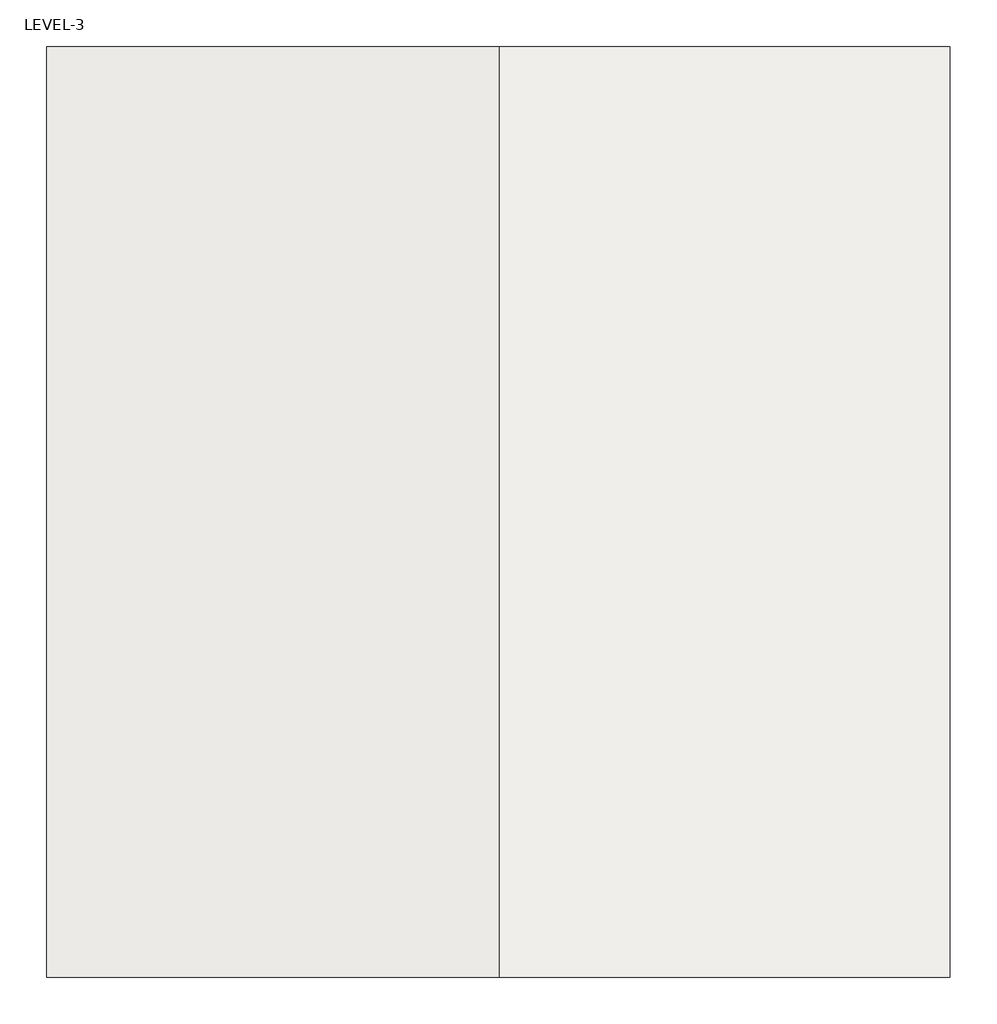
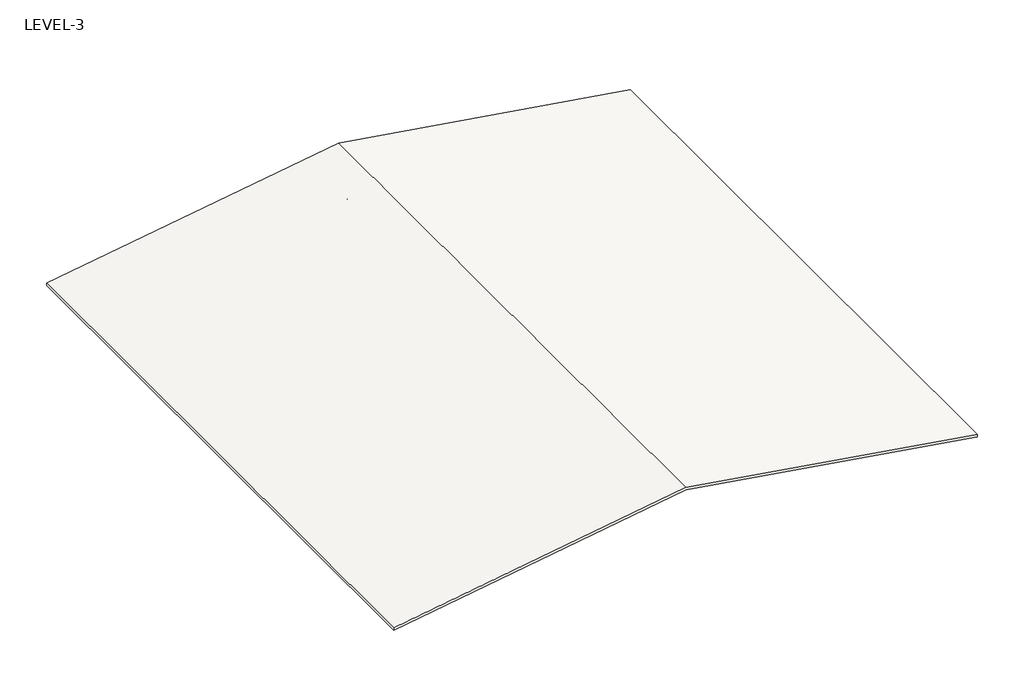
# One storey: 24 beams, 1 roof.
"""IFC4 building model written with IfcOpenShell, lengths in millimetres."""

from ifc_helpers import new_model, si_unit, frame, origin, place, context, project, spatial, polyline, outline, extrude, transform, mapped, element, save
from components import ub_universal_beams_ub305x165x40_7500c72c, ub_universal_beams_ub305x165x40_0b90c1cb, ub_universal_beams_ub305x165x40_52a2f76b, ub_universal_beams_ub305x165x40_7a055ae5

model = new_model("IFC4")

# Units and contexts
model_context = context("Model", 3, world=origin())
ifc_project = project(units=[si_unit("LENGTHUNIT", "METRE", prefix="MILLI")], contexts=[model_context])

# Site, building, storey
site = spatial("IfcSite", under=ifc_project)
building = spatial("IfcBuilding", under=site)
storey = spatial("IfcBuildingStorey", under=building, Name="LEVEL-3", Elevation=6706.0)

# Beams
placement = place(None, origin())
ub_universal_beams_ub305x165x40_shape = ub_universal_beams_ub305x165x40_7500c72c(model_context)
element("IfcBeam", 1, ObjectType="UB-Universal Beams : UB305x165x40", at=placement, inside=storey, context=model_context, shape_type="MappedRepresentation", body=[
    mapped(ub_universal_beams_ub305x165x40_shape, transform((-6850.9138812, -14328.4765895, 5828.2801742), x_axis=(1.0, 0.0, 0.0), y_axis=(0.0, -1.0, 0.0), z_axis=(0.0, 0.0, -1.0))),
])
element("IfcBeam", 2, ObjectType="UB-Universal Beams : UB305x165x40", at=placement, inside=storey, context=model_context, shape_type="MappedRepresentation", body=[
    mapped(ub_universal_beams_ub305x165x40_shape, transform((-6850.9138812, -8232.4765895, 5828.2801742), x_axis=(1.0, 0.0, 0.0), y_axis=(0.0, -1.0, 0.0), z_axis=(0.0, 0.0, -1.0))),
])
element("IfcBeam", 3, ObjectType="UB-Universal Beams : UB305x165x40", at=placement, inside=storey, context=model_context, shape_type="MappedRepresentation", body=[
    mapped(ub_universal_beams_ub305x165x40_shape, transform((-6850.9138812, -2136.4765895, 5828.2801742), x_axis=(1.0, 0.0, 0.0), y_axis=(0.0, -1.0, 0.0), z_axis=(0.0, 0.0, -1.0))),
])
element("IfcBeam", 4, ObjectType="UB-Universal Beams : UB305x165x40", at=placement, inside=storey, context=model_context, shape_type="MappedRepresentation", body=[
    mapped(ub_universal_beams_ub305x165x40_shape, transform((-6850.9138812, 3959.5234105, 5828.2801742), x_axis=(1.0, 0.0, 0.0), y_axis=(0.0, -1.0, 0.0), z_axis=(0.0, 0.0, -1.0))),
])
element("IfcBeam", 5, ObjectType="UB-Universal Beams : UB305x165x40", at=placement, inside=storey, context=model_context, shape_type="MappedRepresentation", body=[
    mapped(ub_universal_beams_ub305x165x40_shape, transform((-6850.9138812, 10055.5234105, 5828.2801742), x_axis=(1.0, 0.0, 0.0), y_axis=(0.0, -1.0, 0.0), z_axis=(0.0, 0.0, -1.0))),
])
element("IfcBeam", 6, ObjectType="UB-Universal Beams : UB305x165x40", at=placement, inside=storey, context=model_context, shape_type="MappedRepresentation", body=[
    mapped(ub_universal_beams_ub305x165x40_shape, transform((-6850.9138812, 16151.5234105, 5828.2801742), x_axis=(1.0, 0.0, 0.0), y_axis=(0.0, -1.0, 0.0), z_axis=(0.0, 0.0, -1.0))),
])
ub_universal_beams_ub305x165x40_2_shape = ub_universal_beams_ub305x165x40_0b90c1cb(model_context)
element("IfcBeam", 7, ObjectType="UB-Universal Beams : UB305x165x40", at=placement, inside=storey, context=model_context, shape_type="MappedRepresentation", body=[
    mapped(ub_universal_beams_ub305x165x40_2_shape, transform((250.2473103, -14328.4765895, 5828.2801742), x_axis=(1.0, 0.0, 0.0), y_axis=(0.0, -1.0, 0.0), z_axis=(0.0, 0.0, -1.0))),
])
element("IfcBeam", 8, ObjectType="UB-Universal Beams : UB305x165x40", at=placement, inside=storey, context=model_context, shape_type="MappedRepresentation", body=[
    mapped(ub_universal_beams_ub305x165x40_2_shape, transform((250.2473103, -8232.4765895, 5828.2801742), x_axis=(1.0, 0.0, 0.0), y_axis=(0.0, -1.0, 0.0), z_axis=(0.0, 0.0, -1.0))),
])
element("IfcBeam", 9, ObjectType="UB-Universal Beams : UB305x165x40", at=placement, inside=storey, context=model_context, shape_type="MappedRepresentation", body=[
    mapped(ub_universal_beams_ub305x165x40_2_shape, transform((250.2473103, -2136.4765895, 5828.2801742), x_axis=(1.0, 0.0, 0.0), y_axis=(0.0, -1.0, 0.0), z_axis=(0.0, 0.0, -1.0))),
])
element("IfcBeam", 10, ObjectType="UB-Universal Beams : UB305x165x40", at=placement, inside=storey, context=model_context, shape_type="MappedRepresentation", body=[
    mapped(ub_universal_beams_ub305x165x40_2_shape, transform((250.2473103, 3959.5234105, 5828.2801742), x_axis=(1.0, 0.0, 0.0), y_axis=(0.0, -1.0, 0.0), z_axis=(0.0, 0.0, -1.0))),
])
element("IfcBeam", 11, ObjectType="UB-Universal Beams : UB305x165x40", at=placement, inside=storey, context=model_context, shape_type="MappedRepresentation", body=[
    mapped(ub_universal_beams_ub305x165x40_2_shape, transform((250.2473103, 10055.5234105, 5828.2801742), x_axis=(1.0, 0.0, 0.0), y_axis=(0.0, -1.0, 0.0), z_axis=(0.0, 0.0, -1.0))),
])
element("IfcBeam", 12, ObjectType="UB-Universal Beams : UB305x165x40", at=placement, inside=storey, context=model_context, shape_type="MappedRepresentation", body=[
    mapped(ub_universal_beams_ub305x165x40_2_shape, transform((250.2473103, 16151.5234105, 5828.2801742), x_axis=(1.0, 0.0, 0.0), y_axis=(0.0, -1.0, 0.0), z_axis=(0.0, 0.0, -1.0))),
])
ub_universal_beams_ub305x165x40_3_shape = ub_universal_beams_ub305x165x40_52a2f76b(model_context)
element("IfcBeam", 13, ObjectType="UB-Universal Beams : UB305x165x40", at=placement, inside=storey, context=model_context, shape_type="MappedRepresentation", body=[
    mapped(ub_universal_beams_ub305x165x40_3_shape, transform((-5118.5854152, -14328.4765895, 6101.0878067), x_axis=(0.15556314184436565, 0.0, -0.9878259507117181), y_axis=(0.0, -1.0, 0.0), z_axis=(-0.9878259507117181, 0.0, -0.15556314184436565))),
])
element("IfcBeam", 14, ObjectType="UB-Universal Beams : UB305x165x40", at=placement, inside=storey, context=model_context, shape_type="MappedRepresentation", body=[
    mapped(ub_universal_beams_ub305x165x40_3_shape, transform((-5118.5854152, -8232.4765895, 6101.0878067), x_axis=(0.15556314184436565, 0.0, -0.9878259507117181), y_axis=(0.0, -1.0, 0.0), z_axis=(-0.9878259507117181, 0.0, -0.15556314184436565))),
])
element("IfcBeam", 15, ObjectType="UB-Universal Beams : UB305x165x40", at=placement, inside=storey, context=model_context, shape_type="MappedRepresentation", body=[
    mapped(ub_universal_beams_ub305x165x40_3_shape, transform((-5118.5854152, -2136.4765895, 6101.0878067), x_axis=(0.15556314184436565, 0.0, -0.9878259507117181), y_axis=(0.0, -1.0, 0.0), z_axis=(-0.9878259507117181, 0.0, -0.15556314184436565))),
])
element("IfcBeam", 16, ObjectType="UB-Universal Beams : UB305x165x40", at=placement, inside=storey, context=model_context, shape_type="MappedRepresentation", body=[
    mapped(ub_universal_beams_ub305x165x40_3_shape, transform((-5118.5854152, 3959.5234105, 6101.0878067), x_axis=(0.15556314184436565, 0.0, -0.9878259507117181), y_axis=(0.0, -1.0, 0.0), z_axis=(-0.9878259507117181, 0.0, -0.15556314184436565))),
])
element("IfcBeam", 17, ObjectType="UB-Universal Beams : UB305x165x40", at=placement, inside=storey, context=model_context, shape_type="MappedRepresentation", body=[
    mapped(ub_universal_beams_ub305x165x40_3_shape, transform((-5118.5854152, 10055.5234105, 6101.0878067), x_axis=(0.15556314184436565, 0.0, -0.9878259507117181), y_axis=(0.0, -1.0, 0.0), z_axis=(-0.9878259507117181, 0.0, -0.15556314184436565))),
])
element("IfcBeam", 18, ObjectType="UB-Universal Beams : UB305x165x40", at=placement, inside=storey, context=model_context, shape_type="MappedRepresentation", body=[
    mapped(ub_universal_beams_ub305x165x40_3_shape, transform((-5118.5854152, 16151.5234105, 6101.0878067), x_axis=(0.15556314184436565, 0.0, -0.9878259507117181), y_axis=(0.0, -1.0, 0.0), z_axis=(-0.9878259507117181, 0.0, -0.15556314184436565))),
])
ub_universal_beams_ub305x165x40_4_shape = ub_universal_beams_ub305x165x40_7a055ae5(model_context)
element("IfcBeam", 19, ObjectType="UB-Universal Beams : UB305x165x40", at=placement, inside=storey, context=model_context, shape_type="MappedRepresentation", body=[
    mapped(ub_universal_beams_ub305x165x40_4_shape, transform((-1482.0811557, -14328.4765895, 6101.0878067), x_axis=(0.15556314184436565, 0.0, 0.9878259507117181), y_axis=(0.0, -1.0, 0.0), z_axis=(0.9878259507117181, 0.0, -0.15556314184436565))),
])
element("IfcBeam", 20, ObjectType="UB-Universal Beams : UB305x165x40", at=placement, inside=storey, context=model_context, shape_type="MappedRepresentation", body=[
    mapped(ub_universal_beams_ub305x165x40_4_shape, transform((-1482.0811557, -8232.4765895, 6101.0878067), x_axis=(0.15556314184436565, 0.0, 0.9878259507117181), y_axis=(0.0, -1.0, 0.0), z_axis=(0.9878259507117181, 0.0, -0.15556314184436565))),
])
element("IfcBeam", 21, ObjectType="UB-Universal Beams : UB305x165x40", at=placement, inside=storey, context=model_context, shape_type="MappedRepresentation", body=[
    mapped(ub_universal_beams_ub305x165x40_4_shape, transform((-1482.0811557, -2136.4765895, 6101.0878067), x_axis=(0.15556314184436565, 0.0, 0.9878259507117181), y_axis=(0.0, -1.0, 0.0), z_axis=(0.9878259507117181, 0.0, -0.15556314184436565))),
])
element("IfcBeam", 22, ObjectType="UB-Universal Beams : UB305x165x40", at=placement, inside=storey, context=model_context, shape_type="MappedRepresentation", body=[
    mapped(ub_universal_beams_ub305x165x40_4_shape, transform((-1482.0811557, 3959.5234105, 6101.0878067), x_axis=(0.15556314184436565, 0.0, 0.9878259507117181), y_axis=(0.0, -1.0, 0.0), z_axis=(0.9878259507117181, 0.0, -0.15556314184436565))),
])
element("IfcBeam", 23, ObjectType="UB-Universal Beams : UB305x165x40", at=placement, inside=storey, context=model_context, shape_type="MappedRepresentation", body=[
    mapped(ub_universal_beams_ub305x165x40_4_shape, transform((-1482.0811557, 10055.5234105, 6101.0878067), x_axis=(0.15556314184436565, 0.0, 0.9878259507117181), y_axis=(0.0, -1.0, 0.0), z_axis=(0.9878259507117181, 0.0, -0.15556314184436565))),
])
element("IfcBeam", 24, ObjectType="UB-Universal Beams : UB305x165x40", at=placement, inside=storey, context=model_context, shape_type="MappedRepresentation", body=[
    mapped(ub_universal_beams_ub305x165x40_4_shape, transform((-1482.0811557, 16151.5234105, 6101.0878067), x_axis=(0.15556314184436565, 0.0, 0.9878259507117181), y_axis=(0.0, -1.0, 0.0), z_axis=(0.9878259507117181, 0.0, -0.15556314184436565))),
])

# Roof
element("IfcRoof", 25, ObjectType="Generic - 400mm", at=placement, inside=storey, context=model_context, shape_type="SweptSolid", body=[
    extrude(outline(polyline([(4066.4394662, -21768.725911), (3912.1612759, -21768.725911), (6821.3093629, -3295.6355591), (3919.6460165, 15129.92669), (4073.9242068, 15129.92669), (6975.5875531, -3295.6355591), (4066.4394662, -21768.725911)])), frame((0.0, -18040.4765895, 0.0), z_axis=(0.0, 1.0, 0.0), x_axis=(0.0, 0.0, 1.0)), (0.0, 0.0, 1.0), 38000.0),
])

save(model, "model.ifc")

# Revit data of these elements
# Type "UB-Universal Beams : UB305x165x40"
#   Section Name Key = "UB305X165X40"
#   Width = 16.5 cm
#   Web Thickness = 0.6 cm
#   Web Fillet = 0.89 cm
#   Warping Constant = 164000.0 cm⁶
#   Torsional Moment of Inertia = 14.70 cm⁴
#   Section Area = 51.3 cm²
#   Plastic Modulus weak axis = 142.0 cm³
#   Plastic Modulus strong axis = 623.0 cm³
#   Nominal Weight = 40.2999 kgf/m
#   Moment of Inertia weak axis = 764.00 cm⁴
#   Moment of Inertia strong axis = 8503.00 cm⁴
#   Height = 30.34 cm
#   Flange Thickness = 1.02 cm
#   Elastic Modulus weak axis = 92.6 cm³
#   Elastic Modulus strong axis = 560.0 cm³
#   Centroid Vertical = 15.17 cm
#   Centroid Horizontal = 8.25 cm
#   Bolt Spacing = 9.0 cm
#   Length [instance default] = 1500 mm
#   Structural Material [instance default] = Metal - Steel 43-275
#   Type Comments = ""
#   Assembly Code = ""
# Type "Generic - 400mm"
#   Layers, outside or top first: 152.4 mm no material (function 1)
# Elements 1, 2, 3, 4, 5, 6, 7, 8, 9, 10, 11, 12, 13, 14, 15, 16, 17, 18, 19, 20, 21, 22, 23, 24 (IfcBeam, "UB-Universal Beams : UB305x165x40")
#   Structural Material = Metal - Steel 43-275
#   Phase Created = New Construction
#   Materials on its faces: "Metal - Steel 43-275"
# Element 25 (IfcRoof, "Generic - 400mm")
#   built-in parameter 1001710 = 33615
#   Phase Created = New Construction
#   Materials on its faces: "Default Roof"
# Materials
#   "Metal - Steel 43-275": class "Metal", colour RGB 247 247 247, transparency 0, Cost = 0
#   "Default Roof": colour RGB 0 127 0, transparency 0, Cost = 0
